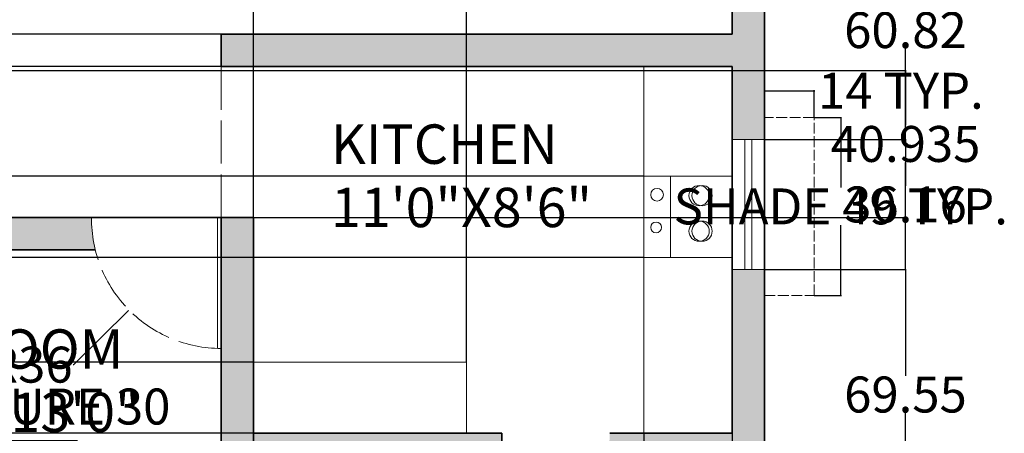
# Model space of a CAD drawing. Units: inches. Extents: x 143 to 746, y -392 to 145.
# Tile 5 of 6: x 473 to 746, y -233 to -118. Entities that reach past the tile are written whole.
import ezdxf

# ---------------------------------------------------------------- set-up
doc = ezdxf.new("R2010")
doc.units = ezdxf.units.IN
doc.header["$MEASUREMENT"] = 0
doc.linetypes.add('ACAD_ISO02W100', pattern=[15, 12, -3])
for name, color, linetype, lineweight in [('A-ANNO-DIMS', 2, 'Continuous', 18), ('A-AREA-IDEN', 7, 'Continuous', 20), ('A-DOOR', 3, 'Continuous', 18), ('A-DOOR-SWNG', 3, 'ACAD_ISO02W100', 13), ('A-EQPM', 8, 'Continuous', 18), ('A-FLOR-CASE', 8, 'Continuous', 20), ('A-GLAZ', 4, 'Continuous', 18), ('A-GLAZ-OVHD', 4, 'ACAD_ISO02W100', 13), ('A-WALL', 7, 'Continuous', 35), ('A-WALL-OVHD', 7, 'ACAD_ISO02W100', 18)]:
    doc.layers.add(name, color=color, linetype=linetype, lineweight=lineweight)
doc.layers.add('A-WALL-PATT', color=252, linetype='Continuous', lineweight=13, true_color=0x939598)
doc.styles.get("Standard").update_dxf_attribs({"font": 'arial.ttf'})
doc.dimstyles.get("Standard").update_dxf_attribs({"dimtxt": 10, "dimasz": 0.18, "dimexe": 0.18, "dimexo": 0.0625, "dimgap": 0.09, "dimtad": 0, "dimtih": 1, "dimtoh": 1, "dimdec": 0, "dimzin": 0, "dimdsep": 46, "dimlunit": 3, "dimtxsty": 'Standard', "dimcen": 0.09, "dimadec": 0, "dimazin": 0, "dimtfac": 1, "dimtdec": 0, "dimtofl": 0, "dimtmove": 0, "dimatfit": 3, "dimfxl": 1, "dimtolj": 1, "dimtzin": 0, "dimarcsym": 0})

# ---------------------------------------------------------------- blocks, each defined once
blk = doc.blocks.new('WINDOW-SHADE-49IN')
at = {"ltscale": 0.25}
for p, q in [((49.48, 13.79), (0, 13.79)), ((0, 13.79), (0, 0)), ((49.48, 0), (49.48, 13.79))]:
    blk.add_line(p, q, dxfattribs=at)
blk = doc.blocks.new('*D12')
at = {"layer": 'A-ANNO-DIMS', "color": 0, "lineweight": -2, "transparency": 16777216}
for p, q in [((369.19, -220.67), (369.19, -225.34)), ((399.54, -220.67), (399.54, -225.34)), ((369.37, -225.16), (399.36, -225.16)), ((399.54, -225.16), (399.72, -225.16))]:
    blk.add_line(p, q, dxfattribs=at)
at = {"layer": 'A-ANNO-DIMS', "color": 0, "transparency": 16777216}
for points in [[(369.37, -225.13), (369.37, -225.19), (369.19, -225.16)], [(399.36, -225.13), (399.36, -225.19), (399.54, -225.16)]]:
    blk.add_solid(points, dxfattribs=at)
at = {"layer": 'Defpoints', "color": 0, "transparency": 16777216}
for p in [(369.19, -220.61), (399.54, -220.61), (399.54, -225.16)]:
    blk.add_point(p, dxfattribs=at)
at = {"layer": 'A-ANNO-DIMS', "color": 0, "transparency": 16777216, "insert": (459.12, -225.16), "char_height": 10, "attachment_point": 5}
blk.add_mtext('\\A1;BATH FIXTURE 30', dxfattribs=at)
blk = doc.blocks.new('*D20')
at = {"layer": 'A-ANNO-DIMS', "color": 0, "lineweight": -2, "transparency": 16777216}
for p, q in [((693.39, -144.77), (700.93, -144.77)), ((700.75, -144.95), (700.75, -164.25)), ((700.75, -194.07), (700.75, -174.77)), ((693.39, -194.25), (700.93, -194.25))]:
    blk.add_line(p, q, dxfattribs=at)
at = {"layer": 'A-ANNO-DIMS', "color": 0, "transparency": 16777216}
for points in [[(700.72, -144.95), (700.78, -144.95), (700.75, -144.77)], [(700.72, -194.07), (700.78, -194.07), (700.75, -194.25)]]:
    blk.add_solid(points, dxfattribs=at)
at = {"layer": 'Defpoints', "color": 0, "transparency": 16777216}
for p in [(693.33, -144.77), (693.33, -194.25), (700.75, -194.25)]:
    blk.add_point(p, dxfattribs=at)
at = {"layer": 'A-ANNO-DIMS', "color": 0, "transparency": 16777216, "insert": (700.75, -169.51), "char_height": 10, "attachment_point": 5}
blk.add_mtext('\\A1;SHADE 49 TYP.', dxfattribs=at)
blk = doc.blocks.new('*D21')
at = {"layer": 'A-ANNO-DIMS', "color": 0, "lineweight": -2, "transparency": 16777216}
for p, q in [((679.54, -144.71), (679.54, -137.17)), ((679.72, -137.35), (693.15, -137.35)), ((693.33, -144.71), (693.33, -137.17)), ((693.33, -137.35), (693.51, -137.35))]:
    blk.add_line(p, q, dxfattribs=at)
at = {"layer": 'A-ANNO-DIMS', "color": 0, "transparency": 16777216}
for points in [[(679.72, -137.32), (679.72, -137.38), (679.54, -137.35)], [(693.15, -137.32), (693.15, -137.38), (693.33, -137.35)]]:
    blk.add_solid(points, dxfattribs=at)
at = {"layer": 'Defpoints', "color": 0, "transparency": 16777216}
for p in [(693.33, -137.35), (679.54, -144.77), (693.33, -144.77)]:
    blk.add_point(p, dxfattribs=at)
at = {"layer": 'A-ANNO-DIMS', "color": 0, "transparency": 16777216, "insert": (717.46, -137.35), "char_height": 10, "attachment_point": 5}
blk.add_mtext('\\A1;14 TYP.', dxfattribs=at)
blk = doc.blocks.new('*D24')
at = {"layer": 'A-ANNO-DIMS', "color": 0, "lineweight": -2, "transparency": 16777216}
for p, q in [((408.54, -234.73), (408.36, -234.73)), ((408.54, -246.67), (408.54, -234.55)), ((488.36, -234.73), (408.72, -234.73)), ((488.54, -246.67), (488.54, -234.55))]:
    blk.add_line(p, q, dxfattribs=at)
at = {"layer": 'A-ANNO-DIMS', "color": 0, "transparency": 16777216}
for points in [[(408.72, -234.7), (408.72, -234.76), (408.54, -234.73)], [(488.36, -234.7), (488.36, -234.76), (488.54, -234.73)]]:
    blk.add_solid(points, dxfattribs=at)
at = {"layer": 'Defpoints', "color": 0, "transparency": 16777216}
for p in [(408.54, -234.73), (408.54, -246.73), (488.54, -246.73)]:
    blk.add_point(p, dxfattribs=at)
at = {"layer": 'A-ANNO-DIMS', "color": 0, "transparency": 16777216, "insert": (340.86, -234.73), "char_height": 10, "attachment_point": 5}
blk.add_mtext('\\A1;QUEEN BED 80 TYP.', dxfattribs=at)
blk = doc.blocks.new('*D44')
at = {"layer": 'A-ANNO-DIMS', "color": 0, "lineweight": -2, "transparency": 16777216}
for p, q in [((189.6, -131.67), (718.91, -131.67)), ((718.73, -131.85), (718.73, -146.94)), ((718.73, -172.43), (718.73, -157.34)), ((198.6, -172.61), (718.91, -172.61))]:
    blk.add_line(p, q, dxfattribs=at)
at = {"layer": 'A-ANNO-DIMS', "color": 0, "transparency": 16777216}
for points in [[(718.7, -131.85), (718.76, -131.85), (718.73, -131.67)], [(718.7, -172.43), (718.76, -172.43), (718.73, -172.61)]]:
    blk.add_solid(points, dxfattribs=at)
at = {"layer": 'Defpoints', "color": 0, "transparency": 16777216}
for p in [(189.54, -131.67), (718.73, -131.67), (198.54, -172.61)]:
    blk.add_point(p, dxfattribs=at)
at = {"layer": 'A-ANNO-DIMS', "color": 0, "transparency": 16777216, "insert": (718.73, -152.14), "char_height": 10, "attachment_point": 5}
blk.add_mtext('\\A1;40.935', dxfattribs=at)
blk = doc.blocks.new('*D59')
at = {"layer": 'A-ANNO-DIMS', "color": 0, "lineweight": -2, "transparency": 16777216}
for p, q in [((679.6, -90.08), (718.91, -90.08)), ((718.73, -90.26), (718.73, -115.29)), ((718.73, -150.71), (718.73, -125.68)), ((679.6, -150.89), (718.91, -150.89))]:
    blk.add_line(p, q, dxfattribs=at)
at = {"layer": 'A-ANNO-DIMS', "color": 0, "transparency": 16777216}
for points in [[(718.7, -90.26), (718.76, -90.26), (718.73, -90.08)], [(718.7, -150.71), (718.76, -150.71), (718.73, -150.89)]]:
    blk.add_solid(points, dxfattribs=at)
at = {"layer": 'Defpoints', "color": 0, "transparency": 16777216}
for p in [(679.54, -90.08), (679.54, -150.89), (718.73, -150.89)]:
    blk.add_point(p, dxfattribs=at)
at = {"layer": 'A-ANNO-DIMS', "color": 0, "transparency": 16777216, "insert": (718.73, -120.48), "char_height": 10, "attachment_point": 5}
blk.add_mtext('\\A1;60.82', dxfattribs=at)
blk = doc.blocks.new('*D60')
at = {"layer": 'A-ANNO-DIMS', "color": 0, "lineweight": -2, "transparency": 16777216}
for p, q in [((679.6, -150.89), (718.91, -150.89)), ((718.73, -151.07), (718.73, -163.77)), ((718.73, -186.87), (718.73, -174.17)), ((679.6, -187.05), (718.91, -187.05))]:
    blk.add_line(p, q, dxfattribs=at)
at = {"layer": 'A-ANNO-DIMS', "color": 0, "transparency": 16777216}
for points in [[(718.7, -151.07), (718.76, -151.07), (718.73, -150.89)], [(718.7, -186.87), (718.76, -186.87), (718.73, -187.05)]]:
    blk.add_solid(points, dxfattribs=at)
at = {"layer": 'Defpoints', "color": 0, "transparency": 16777216}
for p in [(679.54, -150.89), (679.54, -187.05), (718.73, -187.05)]:
    blk.add_point(p, dxfattribs=at)
at = {"layer": 'A-ANNO-DIMS', "color": 0, "transparency": 16777216, "insert": (718.73, -168.97), "char_height": 10, "attachment_point": 5}
blk.add_mtext('\\A1;36.16', dxfattribs=at)
blk = doc.blocks.new('*D61')
at = {"layer": 'A-ANNO-DIMS', "color": 0, "lineweight": -2, "transparency": 16777216}
for p, q in [((679.6, -187.05), (718.91, -187.05)), ((718.73, -187.23), (718.73, -216.63)), ((718.73, -256.42), (718.73, -227.02)), ((679.6, -256.6), (718.91, -256.6))]:
    blk.add_line(p, q, dxfattribs=at)
at = {"layer": 'A-ANNO-DIMS', "color": 0, "transparency": 16777216}
for points in [[(718.7, -187.23), (718.76, -187.23), (718.73, -187.05)], [(718.7, -256.42), (718.76, -256.42), (718.73, -256.6)]]:
    blk.add_solid(points, dxfattribs=at)
at = {"layer": 'Defpoints', "color": 0, "transparency": 16777216}
for p in [(679.54, -187.05), (679.54, -256.6), (718.73, -256.6)]:
    blk.add_point(p, dxfattribs=at)
at = {"layer": 'A-ANNO-DIMS', "color": 0, "transparency": 16777216, "insert": (718.73, -221.82), "char_height": 10, "attachment_point": 5}
blk.add_mtext('\\A1;69.55', dxfattribs=at)
blk = doc.blocks.new('*D64')
at = {"layer": 'A-ANNO-DIMS', "color": 0, "lineweight": -2, "transparency": 16777216}
for p, q in [((646.02, -232.67), (646.02, -385.98)), ((670.54, -232.67), (670.54, -385.98)), ((646.2, -385.8), (670.36, -385.8)), ((670.54, -385.8), (670.72, -385.8))]:
    blk.add_line(p, q, dxfattribs=at)
at = {"layer": 'A-ANNO-DIMS', "color": 0, "transparency": 16777216}
for points in [[(646.2, -385.77), (646.2, -385.83), (646.02, -385.8)], [(670.36, -385.77), (670.36, -385.83), (670.54, -385.8)]]:
    blk.add_solid(points, dxfattribs=at)
at = {"layer": 'Defpoints', "color": 0, "transparency": 16777216}
for p in [(646.02, -232.61), (670.54, -232.61), (670.54, -385.8)]:
    blk.add_point(p, dxfattribs=at)
at = {"layer": 'A-ANNO-DIMS', "color": 0, "transparency": 16777216, "insert": (687.71, -385.8), "char_height": 10, "attachment_point": 5}
blk.add_mtext('\\A1;24.52', dxfattribs=at)
blk = doc.blocks.new('*D65')
at = {"layer": 'A-ANNO-DIMS', "color": 0, "lineweight": -2, "transparency": 16777216}
for p, q in [((537.54, -212.72), (537.54, 139.06)), ((537.72, 138.88), (550.16, 138.88)), ((596.51, 138.88), (584.08, 138.88)), ((596.69, -212.72), (596.69, 139.06))]:
    blk.add_line(p, q, dxfattribs=at)
at = {"layer": 'A-ANNO-DIMS', "color": 0, "transparency": 16777216}
for points in [[(537.72, 138.91), (537.72, 138.85), (537.54, 138.88)], [(596.51, 138.91), (596.51, 138.85), (596.69, 138.88)]]:
    blk.add_solid(points, dxfattribs=at)
at = {"layer": 'Defpoints', "color": 0, "transparency": 16777216}
for p in [(596.69, 138.88), (537.54, -212.78), (596.69, -212.78)]:
    blk.add_point(p, dxfattribs=at)
at = {"layer": 'A-ANNO-DIMS', "color": 0, "transparency": 16777216, "insert": (567.12, 138.88), "char_height": 10, "attachment_point": 5}
blk.add_mtext('\\A1;59.16', dxfattribs=at)
blk = doc.blocks.new('*D66')
at = {"layer": 'A-ANNO-DIMS', "color": 0, "lineweight": -2, "transparency": 16777216}
for p, q in [((537.48, -212.78), (163.96, -212.78)), ((164.14, -212.96), (164.14, -217.49)), ((164.14, -232.43), (164.14, -227.89)), ((537.48, -232.61), (163.96, -232.61))]:
    blk.add_line(p, q, dxfattribs=at)
at = {"layer": 'A-ANNO-DIMS', "color": 0, "transparency": 16777216}
for points in [[(164.11, -212.96), (164.17, -212.96), (164.14, -212.78)], [(164.11, -232.43), (164.17, -232.43), (164.14, -232.61)]]:
    blk.add_solid(points, dxfattribs=at)
at = {"layer": 'Defpoints', "color": 0, "transparency": 16777216}
for p in [(537.54, -212.78), (164.14, -232.61), (537.54, -232.61)]:
    blk.add_point(p, dxfattribs=at)
at = {"layer": 'A-ANNO-DIMS', "color": 0, "transparency": 16777216, "insert": (164.14, -222.69), "char_height": 10, "attachment_point": 5}
blk.add_mtext('\\A1;19.83', dxfattribs=at)
blk = doc.blocks.new('*D67')
at = {"layer": 'A-ANNO-DIMS', "color": 0, "lineweight": -2, "transparency": 16777216}
for p, q in [((528.48, -121.61), (163.96, -121.61)), ((164.14, -121.79), (164.14, -130.43)), ((528.48, -130.61), (163.96, -130.61)), ((164.14, -130.79), (163.96, -130.79)), ((164.14, -130.61), (164.14, -130.79))]:
    blk.add_line(p, q, dxfattribs=at)
at = {"layer": 'A-ANNO-DIMS', "color": 0, "transparency": 16777216}
for points in [[(164.11, -121.79), (164.17, -121.79), (164.14, -121.61)], [(164.11, -130.43), (164.17, -130.43), (164.14, -130.61)]]:
    blk.add_solid(points, dxfattribs=at)
at = {"layer": 'Defpoints', "color": 0, "transparency": 16777216}
for p in [(528.54, -121.61), (164.14, -130.61), (528.54, -130.61)]:
    blk.add_point(p, dxfattribs=at)
at = {"layer": 'A-ANNO-DIMS', "color": 0, "transparency": 16777216, "insert": (160.58, -130.79), "char_height": 10, "attachment_point": 5}
blk.add_mtext('\\A1;9', dxfattribs=at)
blk = doc.blocks.new('*D70')
at = {"layer": 'A-ANNO-DIMS', "color": 0, "lineweight": -2, "transparency": 16777216}
for p, q in [((645.96, -161.14), (163.96, -161.14)), ((164.14, -161.32), (164.14, -167.24)), ((164.14, -183.56), (164.14, -177.64)), ((645.96, -183.74), (163.96, -183.74))]:
    blk.add_line(p, q, dxfattribs=at)
at = {"layer": 'A-ANNO-DIMS', "color": 0, "transparency": 16777216}
for points in [[(164.11, -161.32), (164.17, -161.32), (164.14, -161.14)], [(164.11, -183.56), (164.17, -183.56), (164.14, -183.74)]]:
    blk.add_solid(points, dxfattribs=at)
at = {"layer": 'Defpoints', "color": 0, "transparency": 16777216}
for p in [(646.02, -161.14), (164.14, -183.74), (646.02, -183.74)]:
    blk.add_point(p, dxfattribs=at)
at = {"layer": 'A-ANNO-DIMS', "color": 0, "transparency": 16777216, "insert": (164.14, -172.44), "char_height": 10, "attachment_point": 5}
blk.add_mtext('\\A1;22.604', dxfattribs=at)
blk = doc.blocks.new('*D75')
at = {"layer": 'A-ANNO-DIMS', "color": 0, "lineweight": -2, "transparency": 16777216}
for p, q in [((528.48, -130.61), (163.96, -130.61)), ((164.14, -130.79), (164.14, -146.5)), ((164.14, -172.43), (164.14, -156.72)), ((528.48, -172.61), (163.96, -172.61))]:
    blk.add_line(p, q, dxfattribs=at)
at = {"layer": 'A-ANNO-DIMS', "color": 0, "transparency": 16777216}
for points in [[(164.11, -130.79), (164.17, -130.79), (164.14, -130.61)], [(164.11, -172.43), (164.17, -172.43), (164.14, -172.61)]]:
    blk.add_solid(points, dxfattribs=at)
at = {"layer": 'Defpoints', "color": 0, "transparency": 16777216}
for p in [(164.14, -130.61), (528.54, -130.61), (528.54, -172.61)]:
    blk.add_point(p, dxfattribs=at)
at = {"layer": 'A-ANNO-DIMS', "color": 0, "transparency": 16777216, "insert": (164.14, -151.61), "char_height": 10, "attachment_point": 5}
blk.add_mtext('\\A1;42', dxfattribs=at)
blk = doc.blocks.new('*D77')
at = {"layer": 'A-ANNO-DIMS', "color": 0, "lineweight": -2, "transparency": 16777216}
for p, q in [((528.45, -173), (528.63, -173)), ((528.54, -173.09), (528.54, -172.91)), ((487.58, -213.51), (502.81, -198.45)), ((487.4, -213.51), (487.58, -213.51))]:
    blk.add_line(p, q, dxfattribs=at)
at = {"layer": 'A-ANNO-DIMS', "color": 0, "transparency": 16777216}
blk.add_solid([(502.79, -198.43), (502.83, -198.47), (502.94, -198.32)], dxfattribs=at)
at = {"layer": 'Defpoints', "color": 0, "transparency": 16777216}
for p in [(528.54, -173), (502.94, -198.32)]:
    blk.add_point(p, dxfattribs=at)
at = {"layer": 'A-ANNO-DIMS', "color": 0, "transparency": 16777216, "insert": (475.37, -213.51), "char_height": 10, "attachment_point": 5}
blk.add_mtext('\\A1;R36', dxfattribs=at)

msp = doc.modelspace()

# ---------------------------------------------------------------- hatches: boundary and pattern name
at = {"layer": 'A-WALL-PATT'}
h = msp.add_hatch(color=256, dxfattribs=at)
h.dxf.hatch_style = 1
h.paths.add_polyline_path([(198.538, 19.3924), (257.4275, 19.3924), (257.4275, 28.3924), (189.538, 28.3924), (189.538, -95.6731, -0.06325422), (198.538, -96.8162)])
h.paths.add_polyline_path([(339.538, 66.969), (471.538, 66.969), (472.538, 66.969), (472.538, 31.3924), (472.538, 6.969), (451.2296, 6.969), (451.2296, -2.031), (472.538, -2.031), (472.538, -82.6076), (544.538, -82.6076), (544.538, -38.6894), (535.538, -38.6894), (535.538, -73.6076), (481.538, -73.6076), (481.538, 22.3924), (498.7149, 22.3924), (498.7149, 31.3924), (481.538, 31.3924), (481.538, 66.969), (481.538, 113.4779), (471.538, 113.4779), (471.538, 75.969), (339.538, 75.969), (339.538, 113.4779), (330.538, 113.4779), (330.538, 66.969), (330.538, 28.3924), (293.6446, 28.3924), (293.6446, 19.3924), (330.538, 19.3924), (330.538, 6.969), (330.538, -2.031), (364.5099, -2.031), (364.5099, 6.969), (339.538, 6.969)])
h.paths.add_polyline_path([(570.63, 31.3924), (544.538, 31.3924), (524.7988, 31.3924), (524.7988, 22.3924), (535.538, 22.3924), (535.538, -9.9696, -0.0761882), (544.538, -8.6878), (544.538, 22.3924), (570.63, 22.3924)])
h.paths.add_polyline_path([(679.538, 31.3924), (618.768, 31.3924), (618.768, 22.3924), (670.538, 22.3924), (670.538, -54.5218), (679.538, -54.5218)])
h.paths.add_polyline_path([(679.538, -90.0753), (670.538, -90.0753), (670.538, -121.6076), (537.538, -121.6076), (528.538, -121.6076), (528.538, -130.6076), (537.538, -130.6076), (670.538, -130.6076), (670.538, -150.8923), (679.538, -150.8923)])
h.paths.add_polyline_path([(679.538, -187.0502), (670.538, -187.0502), (670.538, -232.6076), (636.538, -232.6076, -0.07632083), (635.1562, -241.6076), (670.538, -241.6076), (670.538, -256.599), (679.538, -256.599)])
h.paths.add_polyline_path([(606.538, -232.6076), (537.538, -232.6076), (537.538, -241.6076), (597.538, -241.6076), (597.538, -337.6076), (590.545, -337.6076), (590.545, -346.6076), (679.538, -346.6076), (679.538, -316.1251), (670.538, -316.1251), (670.538, -337.6076), (606.538, -337.6076)])
h.paths.add_polyline_path([(537.538, -181.6076), (537.538, -172.6076), (528.538, -172.6076), (528.538, -209.005), (528.538, -269.6672, -0.07632083), (537.538, -271.0491)])
h.paths.add_polyline_path([(566.8252, -337.6076), (537.538, -337.6076), (537.538, -299.6672), (528.538, -299.6672), (528.538, -337.6076), (513.484, -337.6076), (513.484, -346.6076), (566.8252, -346.6076)])
h.paths.add_polyline_path([(477.1278, -337.6076), (408.538, -337.6076), (408.538, -229.6076), (408.538, -181.6076), (493.5793, -181.6076, -0.06316411), (492.538, -172.6076), (399.538, -172.6076), (399.538, -229.6076), (399.538, -337.6076), (388.659, -337.6076), (388.659, -346.6076), (477.1278, -346.6076)])
h.paths.add_polyline_path([(364.4504, -337.6076), (339.538, -337.6076), (339.538, -301.3371), (330.538, -301.3371), (330.538, -337.6076), (307.2736, -337.6076), (307.2736, -346.6076), (364.4504, -346.6076)])
h.paths.add_polyline_path([(339.538, -229.6076), (399.538, -229.6076), (399.538, -220.6076), (369.1898, -220.6076), (330.538, -220.6076), (330.538, -271.2389, -0.07612824), (339.538, -272.6672)])
h.paths.add_polyline_path([(271.3704, -337.6076), (198.538, -337.6076), (198.538, -181.6076), (339.538, -181.6076), (339.538, -172.6076), (198.538, -172.6076), (198.538, -131.6731), (189.538, -131.6731), (189.538, -346.6076), (271.3704, -346.6076)])

# ---------------------------------------------------------------- linework, layer by layer
at = {"layer": 'A-DOOR'}
for p, q in [((527.538, -172.6076), (527.538, -209.005)), ((528.538, -172.6076), (528.538, -209.005)), ((606.538, -232.6076), (606.538, -262.6076))]:
    msp.add_line(p, q, dxfattribs=at)
at = {"layer": 'A-DOOR-SWNG'}
msp.add_arc((528.538, -173.0028), 36.0022, 179.370989, 270, dxfattribs=at)
at = {"layer": 'A-EQPM'}
msp.add_line((653.3987, -161.1374), (653.3987, -183.7414), dxfattribs=at)
msp.add_lwpolyline([(646.0181, -161.1374), (670.538, -161.1374), (670.538, -183.7414), (646.0181, -183.7414)], close=True, dxfattribs=at)
for centre, radius in [((661.3703, -166.5114), 2.8125), ((662.199, -166.5114), 2.8125), ((649.6876, -166.2573), 1.7651), ((649.4225, -175.3477), 1.5004), ((661.3703, -176.4017), 2.8125), ((662.199, -176.4017), 2.8125)]:
    msp.add_circle(centre, radius, dxfattribs=at)
at = {"layer": 'A-FLOR-CASE'}
for p, q in [((646.0181, -232.6076), (646.0181, -130.6076)), ((596.695, -212.7788), (537.538, -212.7788)), ((596.695, -232.6076), (596.695, -212.7788))]:
    msp.add_line(p, q, dxfattribs=at)
at = {"layer": 'A-GLAZ'}
for p, q in [((670.538, -150.8923), (679.538, -150.8923)), ((674.038, -150.8923), (674.038, -187.0502)), ((676.038, -150.8923), (676.038, -187.0502)), ((675.038, -187.0502), (670.538, -187.0502)), ((670.538, -187.0502), (679.538, -187.0502))]:
    msp.add_line(p, q, dxfattribs=at)
at = {"layer": 'A-WALL'}
for p, q in [((679.538, -346.6076), (679.538, 31.3924)), ((670.538, -121.6076), (670.538, 22.3924)), ((537.538, -121.6076), (528.538, -121.6076)), ((528.538, -121.6076), (528.538, -130.6076)), ((670.538, -121.6076), (537.538, -121.6076)), ((528.538, -130.6076), (537.538, -130.6076)), ((670.538, -130.6076), (537.538, -130.6076)), ((670.538, -232.6076), (670.538, -130.6076)), ((679.538, -232.6076), (679.538, -130.6076)), ((492.538, -172.6076), (399.538, -172.6076)), ((537.538, -172.6076), (527.538, -172.6076)), ((528.538, -269.6672), (528.538, -172.6076)), ((537.538, -172.6076), (537.538, -181.6076)), ((493.5793, -181.6076), (408.538, -181.6076)), ((537.538, -271.0491), (537.538, -181.6076)), ((606.538, -232.6076), (537.538, -232.6076)), ((606.538, -337.6076), (606.538, -232.6076)), ((670.538, -232.6076), (636.538, -232.6076))]:
    msp.add_line(p, q, dxfattribs=at)
at = {"layer": 'A-WALL-OVHD'}
for p, q in [((528.538, -130.6076), (528.538, -172.6076)), ((537.538, -172.6076), (537.538, -130.6076))]:
    msp.add_line(p, q, dxfattribs=at)

# ---------------------------------------------------------------- block references
at = {"layer": 'A-GLAZ-OVHD', "rotation": 270}
msp.add_blockref('WINDOW-SHADE-49IN', (679.5376, -144.7717), dxfattribs=at)

# ---------------------------------------------------------------- texts
at = {"layer": 'A-AREA-IDEN'}
for s, height, p in [('KITCHEN', 10.95807, (559.0846, -157.6743)), ('11\'0"X8\'6"', 10.95807, (559.0846, -175.2775)), ('BED ROOM', 10.95807, (425.3066, -214.6495)), ('10\'0"X13\'0"', 10.958074, (425.3066, -232.2526))]:
    msp.add_text(s, height=height, dxfattribs=at).set_placement(p)

# ---------------------------------------------------------------- dimensions: what is measured, and where the dimension line sits
at = {"layer": 'A-ANNO-DIMS'}
for base, p1, p2, picture, middle in [((596.695, 138.8779), (537.538, -212.7788), (596.695, -212.7788), '*D65', (567.1165, 138.8779)), ((670.538, -385.7951), (646.0181, -232.6076), (670.538, -232.6076), '*D64', (687.7146, -385.7951))]:
    dim = msp.add_linear_dim(base=base, p1=p1, p2=p2, dimstyle='Standard', override={"dimdec": 2, "dimlfac": 1, "dimrnd": 0, "dimzin": 0, "dimdsep": 46, "dimlunit": 2}, dxfattribs=at)
    dim.commit()
    dim.dimension.update_dxf_attribs({"geometry": picture, "text_midpoint": middle})
for base, p1, p2, override, picture, middle in [((718.7255, -150.8923), (679.538, -90.0753), (679.538, -150.8923), {"dimdec": 2, "dimlfac": 1, "dimrnd": 0, "dimzin": 0, "dimdsep": 46, "dimlunit": 2}, '*D59', (718.7255, -120.4838)), ((164.138, -130.6076), (528.538, -121.6076), (528.538, -130.6076), {"dimdec": 0, "dimlfac": 1, "dimrnd": 0, "dimzin": 0, "dimdsep": 46, "dimlunit": 2}, '*D67', (160.5802, -130.7876)), ((164.138, -130.6076), (528.538, -172.6076), (528.538, -130.6076), {"dimdec": 0, "dimlfac": 1, "dimrnd": 0, "dimzin": 0, "dimdsep": 46, "dimlunit": 2}, '*D75', (164.138, -151.6076)), ((718.72548, -131.67308), (198.53803, -172.6076), (189.53803, -131.67308), {"dimdec": 3, "dimlfac": 1, "dimrnd": 0, "dimzin": 0, "dimdsep": 46, "dimlunit": 2}, '*D44', (718.72548, -152.14034)), ((718.7255, -187.0502), (679.538, -150.8923), (679.538, -187.0502), {"dimdec": 2, "dimlfac": 1, "dimrnd": 0, "dimzin": 0, "dimdsep": 46, "dimlunit": 2}, '*D60', (718.7255, -168.9713)), ((164.138, -183.7414), (646.0181, -161.1374), (646.0181, -183.7414), {"dimdec": 3, "dimlfac": 1, "dimrnd": 0, "dimzin": 0, "dimdsep": 46, "dimlunit": 2}, '*D70', (164.138, -172.4394)), ((718.7255, -256.599), (679.538, -187.0502), (679.538, -256.599), {"dimdec": 2, "dimlfac": 1, "dimrnd": 0, "dimzin": 0, "dimdsep": 46, "dimlunit": 2}, '*D61', (718.7255, -221.8246)), ((164.138, -232.6076), (537.538, -212.7788), (537.538, -232.6076), {"dimdec": 2, "dimlfac": 1, "dimrnd": 0, "dimzin": 0, "dimdsep": 46, "dimlunit": 2}, '*D66', (164.138, -222.6932))]:
    dim = msp.add_linear_dim(base=base, p1=p1, p2=p2, angle=90, dimstyle='Standard', override=override, dxfattribs=at)
    dim.commit()
    dim.dimension.update_dxf_attribs({"geometry": picture, "text_midpoint": middle})
for base, p1, p2, text, picture, middle in [((693.3255, -137.3493), (679.538, -144.7712), (693.3255, -144.7712), '<> TYP.', '*D21', (717.4631, -137.3493)), ((399.538, -225.1598), (369.1898, -220.6076), (399.538, -220.6076), 'BATH FIXTURE <>', '*D12', (459.1225, -225.1598))]:
    dim = msp.add_linear_dim(base=base, p1=p1, p2=p2, text=text, dimstyle='Standard', override={"dimdec": 0, "dimlfac": 1, "dimrnd": 0, "dimzin": 0, "dimdsep": 46, "dimlunit": 2}, dxfattribs=at)
    dim.commit()
    dim.dimension.update_dxf_attribs({"geometry": picture, "text_midpoint": middle})
for base, p1, p2, angle, text, picture, middle in [((700.7474, -194.2507), (693.3255, -144.7712), (693.3255, -194.2507), 270, 'SHADE <> TYP.', '*D20', (700.7474, -169.511)), ((408.538, -234.7314), (488.5381, -246.7314), (408.538, -246.7314), 180, 'QUEEN BED <> TYP.', '*D24', (340.8567, -234.7314))]:
    dim = msp.add_linear_dim(base=base, p1=p1, p2=p2, angle=angle, text=text, dimstyle='Standard', override={"dimdec": 0, "dimlfac": 1, "dimrnd": 0, "dimzin": 0, "dimdsep": 46, "dimlunit": 2}, dxfattribs=at)
    dim.commit()
    dim.dimension.update_dxf_attribs({"geometry": picture, "text_midpoint": middle})
dim = msp.add_radius_dim(center=(528.538, -173.0028), mpoint=(502.9411, -198.3199), dimstyle='Standard', override={"dimdec": 0, "dimlfac": 1, "dimrnd": 0, "dimzin": 0, "dimdsep": 46, "dimlunit": 2}, dxfattribs=at)
dim.commit()
dim.dimension.update_dxf_attribs({"geometry": '*D77', "text_midpoint": (475.3689, -213.5101), "dimtype": 164})

doc.saveas('drawing.dxf')
